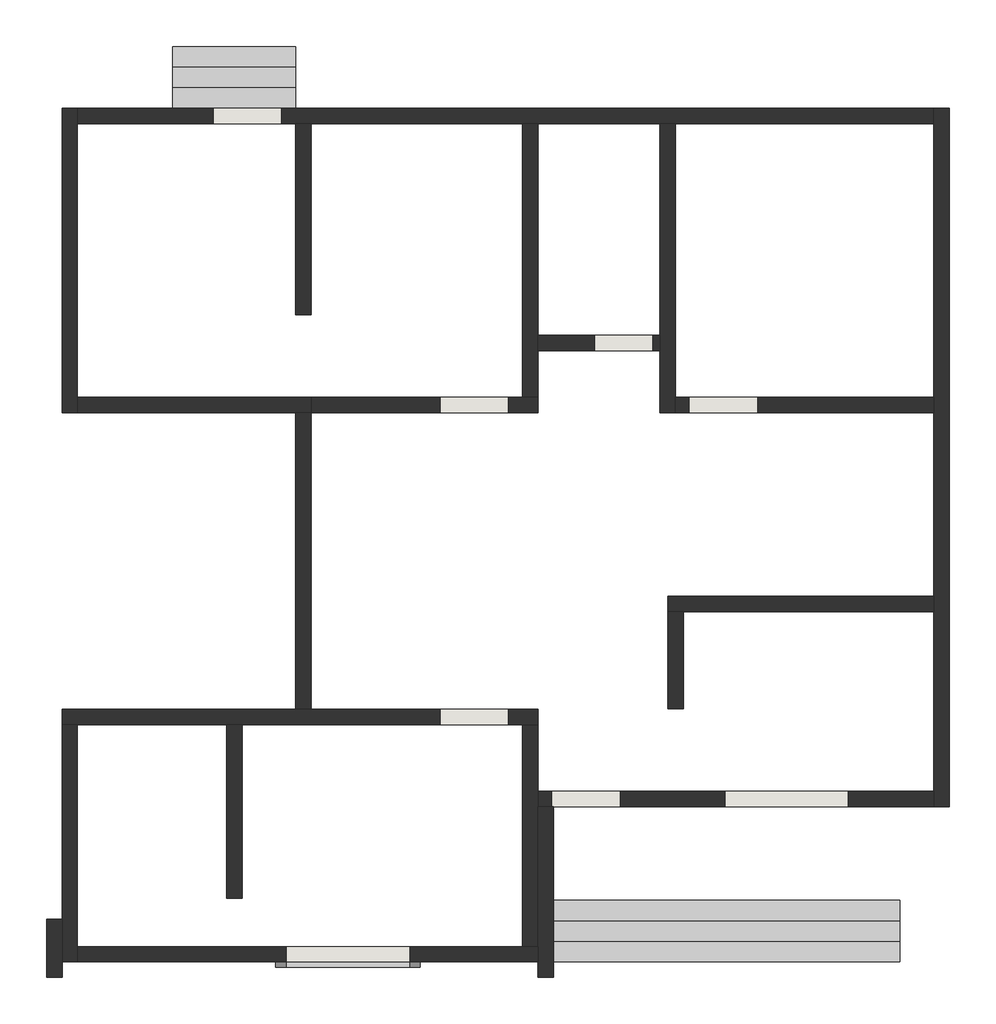
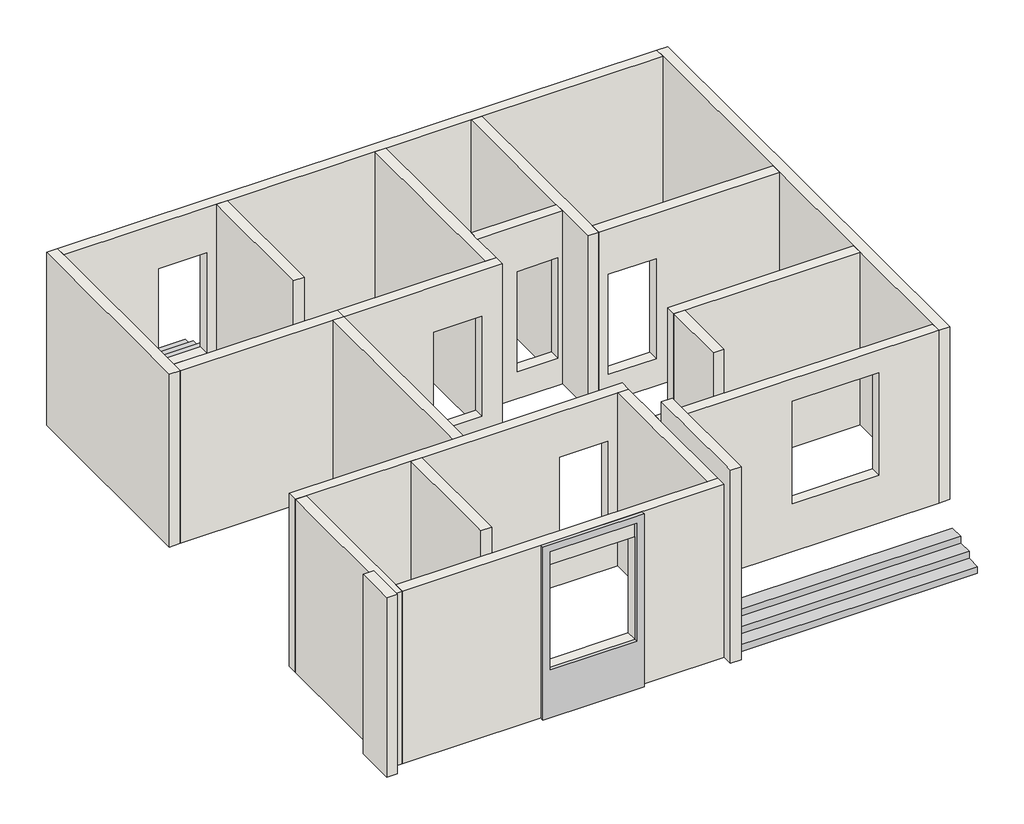
# One storey: 21 walls, 2 stair flights, 1 furniture element.
"""IFC4 building model written with IfcOpenShell, lengths in millimetres."""

from ifc_helpers import new_model, si_unit, frame, origin, origin_with_axes, place, context, project, spatial, polyline, outline, extrude, faceted_brep, transform, mapped, element, save
from components import casework_1_casework_1_6c4e18a6

model = new_model("IFC4")

# Units and contexts
model_context = context("Model", 3, world=origin())
ifc_project = project(units=[si_unit("LENGTHUNIT", "METRE", prefix="MILLI")], contexts=[model_context])

# Site, building, storey
site = spatial("IfcSite", under=ifc_project)
building = spatial("IfcBuilding", under=site)
storey = spatial("IfcBuildingStorey", under=building, Elevation=0.0)

# Furniture
placement = place(None, origin())
casework_1_casework_1_shape = casework_1_casework_1_6c4e18a6(model_context)
element("IfcFurniture", 1, ObjectType="Casework 1 : Casework 1", at=placement, inside=storey, context=model_context, shape_type="MappedRepresentation", body=[
    mapped(casework_1_casework_1_shape, transform((0.0, 0.0, 0.0), x_axis=(1.0, 0.0, 0.0), y_axis=(0.0, 1.0, 0.0), z_axis=(0.0, 0.0, 1.0))),
])

# Stair flights
element("IfcStairFlight", 2, ObjectType="M_Monolithic Run", at=placement, inside=storey, context=model_context, shape_type="Brep", body=[
    faceted_brep([(-13762.7520625, -9926.0480844, 150.0), (-13762.7520625, -10226.0480844, 150.0), (-8495.7520625, -10226.0480844, 150.0), (-8495.7520625, -9926.0480844, 150.0), (-13762.7520625, -9926.0480844, 0.0), (-13762.7520625, -10226.0480844, 0.0), (-8495.7520625, -10226.0480844, 0.0), (-8495.7520625, -9926.0480844, 0.0), (-13762.7520625, -9626.0480844, 300.0), (-13762.7520625, -9926.0480844, 300.0), (-8495.7520625, -9926.0480844, 300.0), (-8495.7520625, -9626.0480844, 300.0), (-13762.7520625, -9626.0480844, 0.0), (-8495.7520625, -9626.0480844, 0.0), (-13762.7520625, -9326.0480844, 450.0), (-13762.7520625, -9626.0480844, 450.0), (-8495.7520625, -9626.0480844, 450.0), (-8495.7520625, -9326.0480844, 450.0), (-13762.7520625, -9326.0480844, 0.0), (-8495.7520625, -9326.0480844, 0.0)], [[[0, 1, 2, 3]], [[1, 0, 4, 5]], [[2, 1, 5, 6]], [[3, 2, 6, 7]], [[8, 9, 10, 11]], [[4, 0, 9, 8, 12]], [[0, 3, 10, 9]], [[3, 7, 13, 11, 10]], [[14, 15, 16, 17]], [[12, 8, 15, 14, 18]], [[8, 11, 16, 15]], [[11, 13, 19, 17, 16]], [[14, 17, 19, 18]], [[5, 4, 12, 18, 19, 13, 7, 6]]]),
])
element("IfcStairFlight", 3, ObjectType="M_Monolithic Run", at=placement, inside=storey, context=model_context, shape_type="Brep", body=[
    faceted_brep([(-17287.7520625, 2790.9519156, 150.0), (-17287.7520625, 3090.9519156, 150.0), (-19074.7520625, 3090.9519156, 150.0), (-19074.7520625, 2790.9519156, 150.0), (-19074.7520625, 3090.9519156, 0.0), (-19074.7520625, 2790.9519156, 0.0), (-17287.7520625, 3090.9519156, 0.0), (-17287.7520625, 2790.9519156, 0.0), (-17287.7520625, 2490.9519156, 300.0), (-17287.7520625, 2790.9519156, 300.0), (-19074.7520625, 2790.9519156, 300.0), (-19074.7520625, 2490.9519156, 300.0), (-19074.7520625, 2490.9519156, 0.0), (-17287.7520625, 2490.9519156, 0.0), (-17287.7520625, 2190.9519156, 450.0), (-17287.7520625, 2490.9519156, 450.0), (-19074.7520625, 2490.9519156, 450.0), (-19074.7520625, 2190.9519156, 450.0), (-19074.7520625, 2190.9519156, 0.0), (-17287.7520625, 2190.9519156, 0.0)], [[[0, 1, 2, 3]], [[3, 2, 4, 5]], [[2, 1, 6, 4]], [[1, 0, 7, 6]], [[8, 9, 10, 11]], [[3, 5, 12, 11, 10]], [[0, 3, 10, 9]], [[7, 0, 9, 8, 13]], [[14, 15, 16, 17]], [[11, 12, 18, 17, 16]], [[8, 11, 16, 15]], [[13, 8, 15, 14, 19]], [[14, 17, 18, 19]], [[6, 7, 13, 19, 18, 12, 5, 4]]]),
])

# Walls
element("IfcWall", 4, ObjectType="01-225 wall", at=placement, inside=storey, context=model_context, shape_type="Brep", body=[
    faceted_brep([(-20687.7520625, 2190.9519156, 0.0), (-20687.7520625, -2234.0480844, 0.0), (-20687.7520625, -2234.0480844, 3800.0), (-20687.7520625, 2190.9519156, 3800.0), (-20462.7520625, 2190.9519156, 0.0), (-20462.7520625, 2190.9519156, 3800.0), (-20462.7520625, 1965.9519156, 3800.0), (-20462.7520625, -2009.0480844, 3800.0), (-20462.7520625, -2234.0480844, 3800.0), (-20462.7520625, -2234.0480844, 0.0), (-20462.7520625, -2009.0480844, 0.0), (-20462.7520625, 1965.9519156, 0.0)], [[[0, 1, 2, 3]], [[4, 5, 6, 7, 8, 9, 10, 11]], [[1, 0, 4, 11, 10, 9]], [[3, 2, 8, 7, 6, 5]], [[0, 3, 5, 4]], [[2, 1, 9, 8]]]),
])
element("IfcWall", 5, ObjectType="01-225 wall", at=placement, inside=storey, context=model_context, shape_type="Brep", body=[
    faceted_brep([(-20462.7520625, -10226.0480844, 0.0), (-13762.7520625, -10226.0480844, 0.0), (-13762.7520625, -10226.0480844, 3800.0), (-20462.7520625, -10226.0480844, 3800.0), (-17425.2520625, -10226.0480844, 1050.0), (-17425.2520625, -10226.0480844, 3300.0), (-15625.2520625, -10226.0480844, 3300.0), (-15625.2520625, -10226.0480844, 1050.0), (-13762.7520625, -10001.0480844, 0.0), (-13987.7520625, -10001.0480844, 0.0), (-20462.7520625, -10001.0480844, 0.0), (-20462.7520625, -10001.0480844, 3800.0), (-13987.7520625, -10001.0480844, 3800.0), (-13762.7520625, -10001.0480844, 3800.0), (-17425.2520625, -10001.0480844, 3300.0), (-17425.2520625, -10001.0480844, 1050.0), (-15625.2520625, -10001.0480844, 1050.0), (-15625.2520625, -10001.0480844, 3300.0)], [[[0, 1, 2, 3], [4, 5, 6, 7]], [[8, 9, 10, 11, 12, 13], [14, 15, 16, 17]], [[1, 0, 10, 9, 8]], [[3, 2, 13, 12, 11]], [[0, 3, 11, 10]], [[2, 1, 8, 13]], [[4, 15, 14, 5]], [[5, 14, 17, 6]], [[6, 17, 16, 7]], [[15, 4, 7, 16]]]),
])
element("IfcWall", 6, ObjectType="01-225 wall", at=placement, inside=storey, context=model_context, shape_type="Brep", body=[
    faceted_brep([(-7770.7520625, -7966.0480844, 0.0), (-7770.7520625, 2190.9519156, 0.0), (-7770.7520625, 2190.9519156, 3800.0), (-7770.7520625, -7966.0480844, 3800.0), (-7995.7520625, -7966.0480844, 0.0), (-7995.7520625, -7966.0480844, 3800.0), (-7995.7520625, -7741.0480844, 3800.0), (-7995.7520625, -5134.0480844, 3800.0), (-7995.7520625, -4909.0480844, 3800.0), (-7995.7520625, -2234.0480844, 3800.0), (-7995.7520625, -2009.0480844, 3800.0), (-7995.7520625, 1965.9519156, 3800.0), (-7995.7520625, 2190.9519156, 3800.0), (-7995.7520625, 2190.9519156, 0.0), (-7995.7520625, 1965.9519156, 0.0), (-7995.7520625, -2009.0480844, 0.0), (-7995.7520625, -2234.0480844, 0.0), (-7995.7520625, -4909.0480844, 0.0), (-7995.7520625, -5134.0480844, 0.0), (-7995.7520625, -7741.0480844, 0.0)], [[[0, 1, 2, 3]], [[4, 5, 6, 7, 8, 9, 10, 11, 12, 13, 14, 15, 16, 17, 18, 19]], [[1, 0, 4, 19, 18, 17, 16, 15, 14, 13]], [[3, 2, 12, 11, 10, 9, 8, 7, 6, 5]], [[2, 1, 13, 12]], [[0, 3, 5, 4]]]),
])
element("IfcWall", 7, ObjectType="01-225 wall", at=placement, inside=storey, context=model_context, shape_type="Brep", body=[
    faceted_brep([(-7995.7520625, 2190.9519156, 0.0), (-20462.7520625, 2190.9519156, 0.0), (-20462.7520625, 2190.9519156, 3800.0), (-7995.7520625, 2190.9519156, 3800.0), (-17487.7520625, 2190.9519156, 600.0), (-17487.7520625, 2190.9519156, 2800.0), (-18487.7520625, 2190.9519156, 2800.0), (-18487.7520625, 2190.9519156, 600.0), (-7995.7520625, 1965.9519156, 0.0), (-7995.7520625, 1965.9519156, 3800.0), (-11762.7520625, 1965.9519156, 3800.0), (-11987.7520625, 1965.9519156, 3800.0), (-13762.7520625, 1965.9519156, 3800.0), (-13987.7520625, 1965.9519156, 3800.0), (-17062.7520625, 1965.9519156, 3800.0), (-17287.7520625, 1965.9519156, 3800.0), (-20462.7520625, 1965.9519156, 3800.0), (-20462.7520625, 1965.9519156, 0.0), (-17287.7520625, 1965.9519156, 0.0), (-17062.7520625, 1965.9519156, 0.0), (-13987.7520625, 1965.9519156, 0.0), (-13762.7520625, 1965.9519156, 0.0), (-11987.7520625, 1965.9519156, 0.0), (-11762.7520625, 1965.9519156, 0.0), (-17487.7520625, 1965.9519156, 600.0), (-18487.7520625, 1965.9519156, 600.0), (-18487.7520625, 1965.9519156, 2800.0), (-17487.7520625, 1965.9519156, 2800.0)], [[[0, 1, 2, 3], [4, 5, 6, 7]], [[8, 9, 10, 11, 12, 13, 14, 15, 16, 17, 18, 19, 20, 21, 22, 23], [24, 25, 26, 27]], [[1, 0, 8, 23, 22, 21, 20, 19, 18, 17]], [[3, 2, 16, 15, 14, 13, 12, 11, 10, 9]], [[2, 1, 17, 16]], [[0, 3, 9, 8]], [[5, 4, 24, 27]], [[6, 5, 27, 26]], [[7, 6, 26, 25]], [[4, 7, 25, 24]]]),
])
element("IfcWall", 8, ObjectType="01-225 wall", at=placement, inside=storey, context=model_context, shape_type="SweptSolid", body=[
    extrude(outline(polyline([(-17287.7520625, -809.0480844), (-17287.7520625, 1965.9519156), (-17062.7520625, 1965.9519156), (-17062.7520625, -809.0480844), (-17287.7520625, -809.0480844)])), origin_with_axes(), (0.0, 0.0, 1.0), 3800.0),
])
element("IfcWall", 9, ObjectType="01-225 wall", at=placement, inside=storey, context=model_context, shape_type="Brep", body=[
    faceted_brep([(-17062.7520625, -2009.0480844, 0.0), (-20462.7520625, -2009.0480844, 0.0), (-20462.7520625, -2009.0480844, 3800.0), (-17062.7520625, -2009.0480844, 3800.0), (-17062.7520625, -2234.0480844, 0.0), (-17062.7520625, -2234.0480844, 3800.0), (-17287.7520625, -2234.0480844, 3800.0), (-20462.7520625, -2234.0480844, 3800.0), (-20462.7520625, -2234.0480844, 0.0), (-17287.7520625, -2234.0480844, 0.0)], [[[0, 1, 2, 3]], [[4, 5, 6, 7, 8, 9]], [[1, 0, 4, 9, 8]], [[3, 2, 7, 6, 5]], [[0, 3, 5, 4]], [[2, 1, 8, 7]]]),
])
element("IfcWall", 10, ObjectType="01-225 wall", at=placement, inside=storey, context=model_context, shape_type="Brep", body=[
    faceted_brep([(-13762.7520625, -6549.0480844, 0.0), (-17062.7520625, -6549.0480844, 0.0), (-17287.7520625, -6549.0480844, 0.0), (-20687.7520625, -6549.0480844, 0.0), (-20687.7520625, -6549.0480844, 3800.0), (-17287.7520625, -6549.0480844, 3800.0), (-17062.7520625, -6549.0480844, 3800.0), (-13762.7520625, -6549.0480844, 3800.0), (-14187.7520625, -6549.0480844, 600.0), (-14187.7520625, -6549.0480844, 2800.0), (-15187.7520625, -6549.0480844, 2800.0), (-15187.7520625, -6549.0480844, 600.0), (-13762.7520625, -6774.0480844, 0.0), (-13762.7520625, -6774.0480844, 3800.0), (-13987.7520625, -6774.0480844, 3800.0), (-18062.7520625, -6774.0480844, 3800.0), (-18287.7520625, -6774.0480844, 3800.0), (-20462.7520625, -6774.0480844, 3800.0), (-20687.7520625, -6774.0480844, 3800.0), (-20687.7520625, -6774.0480844, 0.0), (-20462.7520625, -6774.0480844, 0.0), (-18287.7520625, -6774.0480844, 0.0), (-18062.7520625, -6774.0480844, 0.0), (-13987.7520625, -6774.0480844, 0.0), (-14187.7520625, -6774.0480844, 600.0), (-15187.7520625, -6774.0480844, 600.0), (-15187.7520625, -6774.0480844, 2800.0), (-14187.7520625, -6774.0480844, 2800.0)], [[[0, 1, 2, 3, 4, 5, 6, 7], [8, 9, 10, 11]], [[12, 13, 14, 15, 16, 17, 18, 19, 20, 21, 22, 23], [24, 25, 26, 27]], [[3, 2, 1, 0, 12, 23, 22, 21, 20, 19]], [[7, 6, 5, 4, 18, 17, 16, 15, 14, 13]], [[0, 7, 13, 12]], [[9, 8, 24, 27]], [[10, 9, 27, 26]], [[11, 10, 26, 25]], [[8, 11, 25, 24]], [[4, 3, 19, 18]]]),
])
element("IfcWall", 11, ObjectType="01-225 wall", at=placement, inside=storey, context=model_context, shape_type="Brep", body=[
    faceted_brep([(-18287.7520625, -6774.0480844, 0.0), (-18287.7520625, -9301.0480844, 0.0), (-18287.7520625, -9301.0480844, 3800.0), (-18287.7520625, -8601.0480844, 3800.0), (-18287.7520625, -8451.0480844, 3800.0), (-18287.7520625, -6774.0480844, 3800.0), (-18062.7520625, -6774.0480844, 0.0), (-18062.7520625, -6774.0480844, 3800.0), (-18062.7520625, -9301.0480844, 3800.0), (-18062.7520625, -9301.0480844, 0.0)], [[[0, 1, 2, 3, 4, 5]], [[6, 7, 8, 9]], [[1, 0, 6, 9]], [[2, 1, 9, 8]], [[5, 4, 3, 2, 8, 7]], [[0, 5, 7, 6]]]),
])
element("IfcWall", 12, ObjectType="01-225 wall", at=placement, inside=storey, context=model_context, shape_type="Brep", body=[
    faceted_brep([(-13987.7520625, -6774.0480844, 0.0), (-13987.7520625, -10001.0480844, 0.0), (-13987.7520625, -10001.0480844, 3800.0), (-13987.7520625, -6774.0480844, 3800.0), (-13762.7520625, -6774.0480844, 0.0), (-13762.7520625, -6774.0480844, 3800.0), (-13762.7520625, -7741.0480844, 3800.0), (-13762.7520625, -7966.0480844, 3800.0), (-13762.7520625, -10001.0480844, 3800.0), (-13762.7520625, -10001.0480844, 0.0), (-13762.7520625, -7966.0480844, 0.0), (-13762.7520625, -7741.0480844, 0.0)], [[[0, 1, 2, 3]], [[4, 5, 6, 7, 8, 9, 10, 11]], [[1, 0, 4, 11, 10, 9]], [[3, 2, 8, 7, 6, 5]], [[0, 3, 5, 4]], [[2, 1, 9, 8]]]),
])
element("IfcWall", 13, ObjectType="01-225 wall", at=placement, inside=storey, context=model_context, shape_type="Brep", body=[
    faceted_brep([(-7995.7520625, -7741.0480844, 0.0), (-13762.7520625, -7741.0480844, 0.0), (-13762.7520625, -7741.0480844, 3800.0), (-7995.7520625, -7741.0480844, 3800.0), (-13562.7520625, -7741.0480844, 600.0), (-12562.7520625, -7741.0480844, 600.0), (-12562.7520625, -7741.0480844, 2800.0), (-13562.7520625, -7741.0480844, 2800.0), (-11042.7520625, -7741.0480844, 3300.0), (-11042.7520625, -7741.0480844, 1050.0), (-9242.7520625, -7741.0480844, 1050.0), (-9242.7520625, -7741.0480844, 3300.0), (-13762.7520625, -7966.0480844, 0.0), (-13537.7520625, -7966.0480844, 0.0), (-7995.7520625, -7966.0480844, 0.0), (-7995.7520625, -7966.0480844, 3800.0), (-13762.7520625, -7966.0480844, 3800.0), (-13562.7520625, -7966.0480844, 600.0), (-13562.7520625, -7966.0480844, 2800.0), (-12562.7520625, -7966.0480844, 2800.0), (-12562.7520625, -7966.0480844, 600.0), (-11042.7520625, -7966.0480844, 1050.0), (-11042.7520625, -7966.0480844, 3300.0), (-9242.7520625, -7966.0480844, 3300.0), (-9242.7520625, -7966.0480844, 1050.0)], [[[0, 1, 2, 3], [4, 5, 6, 7], [8, 9, 10, 11]], [[12, 13, 14, 15, 16], [17, 18, 19, 20], [21, 22, 23, 24]], [[1, 0, 14, 13, 12]], [[3, 2, 16, 15]], [[2, 1, 12, 16]], [[0, 3, 15, 14]], [[18, 17, 4, 7]], [[19, 18, 7, 6]], [[20, 19, 6, 5]], [[17, 20, 5, 4]], [[21, 9, 8, 22]], [[22, 8, 11, 23]], [[23, 11, 10, 24]], [[9, 21, 24, 10]]]),
])
element("IfcWall", 14, ObjectType="01-225 wall", at=placement, inside=storey, context=model_context, shape_type="Brep", body=[
    faceted_brep([(-7995.7520625, -4909.0480844, 0.0), (-11867.7520625, -4909.0480844, 0.0), (-11867.7520625, -4909.0480844, 3800.0), (-7995.7520625, -4909.0480844, 3800.0), (-7995.7520625, -5134.0480844, 0.0), (-7995.7520625, -5134.0480844, 3800.0), (-11642.7520625, -5134.0480844, 3800.0), (-11867.7520625, -5134.0480844, 3800.0), (-11867.7520625, -5134.0480844, 0.0), (-11642.7520625, -5134.0480844, 0.0)], [[[0, 1, 2, 3]], [[4, 5, 6, 7, 8, 9]], [[1, 0, 4, 9, 8]], [[3, 2, 7, 6, 5]], [[0, 3, 5, 4]], [[2, 1, 8, 7]]]),
])
element("IfcWall", 15, ObjectType="01-225 wall", at=placement, inside=storey, context=model_context, shape_type="SweptSolid", body=[
    extrude(outline(polyline([(-11867.7520625, -6541.0480844), (-11867.7520625, -5134.0480844), (-11642.7520625, -5134.0480844), (-11642.7520625, -6541.0480844), (-11867.7520625, -6541.0480844)])), origin_with_axes(), (0.0, 0.0, 1.0), 3800.0),
])
element("IfcWall", 16, ObjectType="01-225 wall", at=placement, inside=storey, context=model_context, shape_type="Brep", body=[
    faceted_brep([(-13987.7520625, 1965.9519156, 0.0), (-13987.7520625, -2009.0480844, 0.0), (-13987.7520625, -2009.0480844, 3800.0), (-13987.7520625, 1965.9519156, 3800.0), (-13762.7520625, 1965.9519156, 0.0), (-13762.7520625, 1965.9519156, 3800.0), (-13762.7520625, -1109.0480844, 3800.0), (-13762.7520625, -1334.0480844, 3800.0), (-13762.7520625, -2009.0480844, 3800.0), (-13762.7520625, -2009.0480844, 0.0), (-13762.7520625, -1334.0480844, 0.0), (-13762.7520625, -1109.0480844, 0.0)], [[[0, 1, 2, 3]], [[4, 5, 6, 7, 8, 9, 10, 11]], [[1, 0, 4, 11, 10, 9]], [[3, 2, 8, 7, 6, 5]], [[0, 3, 5, 4]], [[2, 1, 9, 8]]]),
])
element("IfcWall", 17, ObjectType="01-225 wall", at=placement, inside=storey, context=model_context, shape_type="SweptSolid", body=[
    extrude(outline(polyline([(0.0, -13762.7520625), (0.0, -11987.7520625), (3800.0, -11987.7520625), (3800.0, -13762.7520625), (0.0, -13762.7520625)]), holes=[polyline([(600.0, -12087.7520625), (600.0, -12937.7520625), (2800.0, -12937.7520625), (2800.0, -12087.7520625), (600.0, -12087.7520625)])]), frame((0.0, -1334.0480844, 0.0), z_axis=(0.0, 1.0, 0.0), x_axis=(0.0, 0.0, 1.0)), (0.0, 0.0, 1.0), 225.0),
])
element("IfcWall", 18, ObjectType="01-225 wall", at=placement, inside=storey, context=model_context, shape_type="Brep", body=[
    faceted_brep([(-11762.7520625, -2234.0480844, 0.0), (-11762.7520625, -2009.0480844, 0.0), (-11762.7520625, 1965.9519156, 0.0), (-11762.7520625, 1965.9519156, 3800.0), (-11762.7520625, -2009.0480844, 3800.0), (-11762.7520625, -2234.0480844, 3800.0), (-11987.7520625, -2234.0480844, 0.0), (-11987.7520625, -2234.0480844, 3800.0), (-11987.7520625, -1334.0480844, 3800.0), (-11987.7520625, -1109.0480844, 3800.0), (-11987.7520625, 1965.9519156, 3800.0), (-11987.7520625, 1965.9519156, 0.0), (-11987.7520625, -1109.0480844, 0.0), (-11987.7520625, -1334.0480844, 0.0)], [[[0, 1, 2, 3, 4, 5]], [[6, 7, 8, 9, 10, 11, 12, 13]], [[2, 1, 0, 6, 13, 12, 11]], [[5, 4, 3, 10, 9, 8, 7]], [[3, 2, 11, 10]], [[0, 5, 7, 6]]]),
])
element("IfcWall", 19, ObjectType="01-225 wall", at=placement, inside=storey, context=model_context, shape_type="Brep", body=[
    faceted_brep([(-17062.7520625, -2234.0480844, 0.0), (-13762.7520625, -2234.0480844, 0.0), (-13762.7520625, -2234.0480844, 3800.0), (-17062.7520625, -2234.0480844, 3800.0), (-14187.7520625, -2234.0480844, 600.0), (-15187.7520625, -2234.0480844, 600.0), (-15187.7520625, -2234.0480844, 2800.0), (-14187.7520625, -2234.0480844, 2800.0), (-17062.7520625, -2009.0480844, 0.0), (-17062.7520625, -2009.0480844, 3800.0), (-13987.7520625, -2009.0480844, 3800.0), (-13762.7520625, -2009.0480844, 3800.0), (-13762.7520625, -2009.0480844, 0.0), (-13987.7520625, -2009.0480844, 0.0), (-14187.7520625, -2009.0480844, 600.0), (-14187.7520625, -2009.0480844, 2800.0), (-15187.7520625, -2009.0480844, 2800.0), (-15187.7520625, -2009.0480844, 600.0)], [[[0, 1, 2, 3], [4, 5, 6, 7]], [[8, 9, 10, 11, 12, 13], [14, 15, 16, 17]], [[1, 0, 8, 13, 12]], [[3, 2, 11, 10, 9]], [[0, 3, 9, 8]], [[2, 1, 12, 11]], [[15, 14, 4, 7]], [[16, 15, 7, 6]], [[17, 16, 6, 5]], [[14, 17, 5, 4]]]),
])
element("IfcWall", 20, ObjectType="01-225 wall", at=placement, inside=storey, context=model_context, shape_type="SweptSolid", body=[
    extrude(outline(polyline([(0.0, -11762.7520625), (0.0, -7995.7520625), (3800.0, -7995.7520625), (3800.0, -11762.7520625), (0.0, -11762.7520625)]), holes=[polyline([(600.0, -11562.7520625), (2800.0, -11562.7520625), (2800.0, -10562.7520625), (600.0, -10562.7520625), (600.0, -11562.7520625)])]), frame((0.0, -2234.0480844, 0.0), z_axis=(0.0, 1.0, 0.0), x_axis=(0.0, 0.0, 1.0)), (0.0, 0.0, 1.0), 225.0),
])
element("IfcWall", 21, ObjectType="01-225 wall", at=placement, inside=storey, context=model_context, shape_type="SweptSolid", body=[
    extrude(outline(polyline([(-17287.7520625, -6549.0480844), (-17287.7520625, -2234.0480844), (-17062.7520625, -2234.0480844), (-17062.7520625, -6549.0480844), (-17287.7520625, -6549.0480844)])), origin_with_axes(), (0.0, 0.0, 1.0), 3800.0),
])
element("IfcWall", 22, ObjectType="01-225 wall", at=placement, inside=storey, context=model_context, shape_type="Brep", body=[
    faceted_brep([(-20687.7520625, -6774.0480844, 0.0), (-20687.7520625, -10226.0480844, 0.0), (-20687.7520625, -10226.0480844, 3800.0), (-20687.7520625, -6774.0480844, 3800.0), (-20462.7520625, -6774.0480844, 0.0), (-20462.7520625, -6774.0480844, 3800.0), (-20462.7520625, -8451.0480844, 3800.0), (-20462.7520625, -8601.0480844, 3800.0), (-20462.7520625, -10001.0480844, 3800.0), (-20462.7520625, -10226.0480844, 3800.0), (-20462.7520625, -10226.0480844, 0.0), (-20462.7520625, -10001.0480844, 0.0)], [[[0, 1, 2, 3]], [[4, 5, 6, 7, 8, 9, 10, 11]], [[1, 0, 4, 11, 10]], [[3, 2, 9, 8, 7, 6, 5]], [[2, 1, 10, 9]], [[0, 3, 5, 4]]]),
])
element("IfcWall", 23, ObjectType="01-225 wall", at=placement, inside=storey, context=model_context, shape_type="Brep", body=[
    faceted_brep([(-13762.7520625, -7966.0480844, 4250.0), (-13762.7520625, -7966.0480844, 3800.0), (-13762.7520625, -7966.0480844, 0.0), (-13762.7520625, -10451.0480844, 0.0), (-13762.7520625, -10451.0480844, 3950.0), (-13762.7520625, -10451.0480844, 4250.0), (-13762.7520625, -10226.0480844, 4250.0), (-13537.7520625, -7966.0480844, 0.0), (-13537.7520625, -7966.0480844, 4250.0), (-13537.7520625, -10451.0480844, 4250.0), (-13537.7520625, -10451.0480844, 0.0)], [[[0, 1, 2, 3, 4, 5, 6]], [[7, 8, 9, 10]], [[3, 2, 7, 10]], [[5, 4, 3, 10, 9]], [[0, 6, 5, 9, 8]], [[0, 8, 7, 2, 1]]]),
])
element("IfcWall", 24, ObjectType="01-225 wall", at=placement, inside=storey, context=model_context, shape_type="SweptSolid", body=[
    extrude(outline(polyline([(-20912.7520625, -10451.0480844), (-20912.7520625, -9601.0480844), (-20687.7520625, -9601.0480844), (-20687.7520625, -10451.0480844), (-20912.7520625, -10451.0480844)])), origin_with_axes(), (0.0, 0.0, 1.0), 3950.0),
])

save(model, "model.ifc")

# Revit data of these elements
# Type "01-225 wall"
#   Description = "Generic Wall (Material By Category), 200mm thick"
#   Assembly Code = "B2010"
#   Type Mark = "G06"
#   Layers, outside or top first: 225 mm "01-225 main wall" (function 1)
# Element 1 (IfcFurniture, "Casework 1 : Casework 1")
#   Phase Created = New Construction
# Elements 2, 3 (IfcStairFlight, "M_Monolithic Run")
#   Phase Created = New Construction
#   Materials on its faces: "00-steps"
# Elements 4, 5, 6, 7, 8, 9, 10, 11, 12, 13, 14, 15, 16, 17, 18, 19, 20, 21, 22 (IfcWall, "01-225 wall")
#   Top Offset = 0 mm
#   Base Offset = 0 mm
#   wall height = 3800 mm
#   Phase Created = New Construction
#   Base Constraint = 0-NFL
#   Top Constraint = 03-first floor
#   Materials on its faces: "01-225 main wall"
# Element 23 (IfcWall, "01-225 wall")
#   Top Offset = 950 mm
#   Base Offset = 0 mm
#   wall height = 4250 mm
#   Phase Created = New Construction
#   Base Constraint = 0-NFL
#   Materials on its faces: "01-225 main wall"
# Element 24 (IfcWall, "01-225 wall")
#   Top Offset = 650 mm
#   Base Offset = 0 mm
#   wall height = 3950 mm
#   Phase Created = New Construction
#   Base Constraint = 0-NFL
#   Materials on its faces: "01-225 main wall"
# Materials
#   "01-225 main wall": class "Generic", colour RGB 244 244 244, transparency 0, Cost = 0
#   "00-steps": class "Generic", colour RGB 120 120 120, transparency 0, Cost = 0
